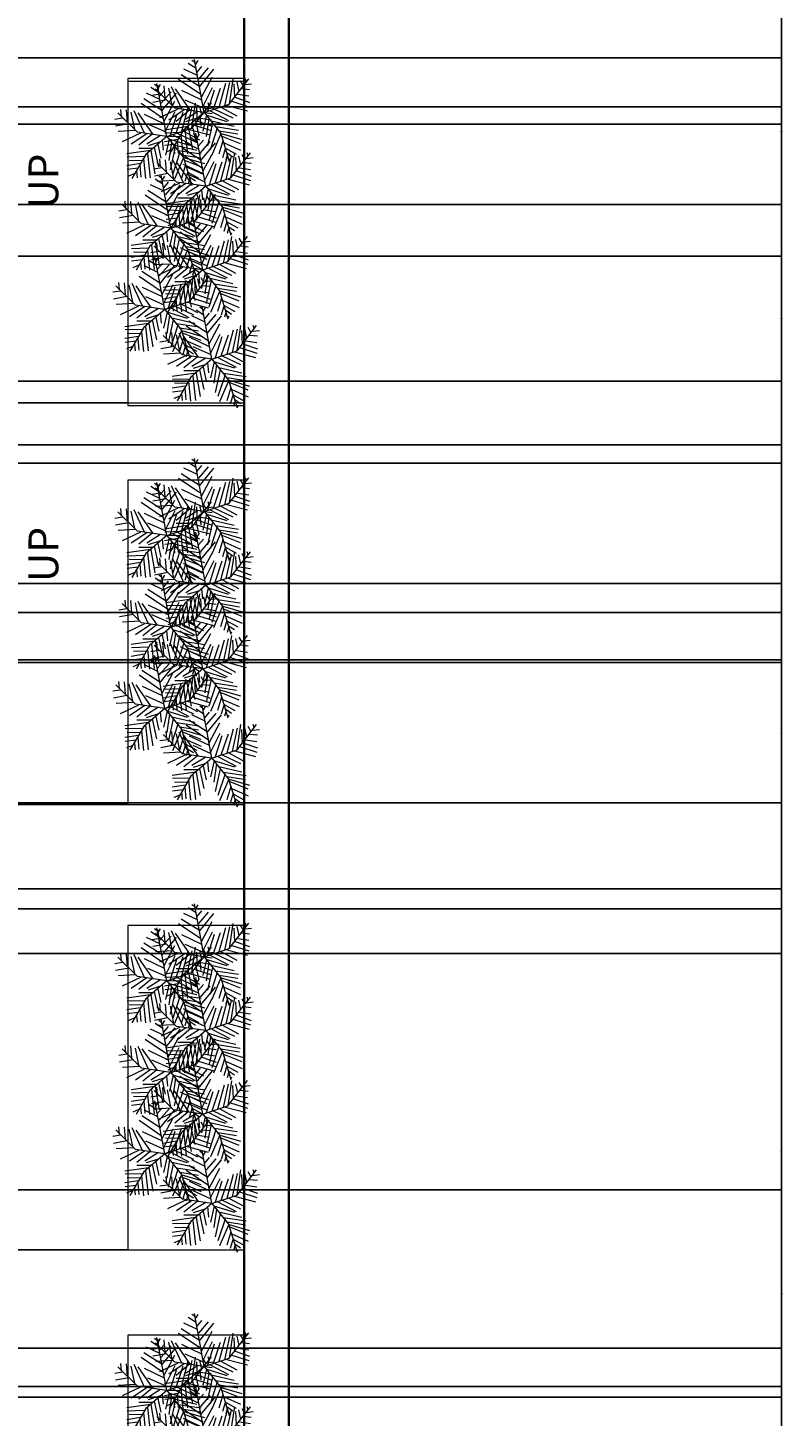
# Model space of a CAD drawing. Units: inches. Extents: x 818 to 1898, y 976 to 2364.
# Tile 56 of 96: x 1746 to 1898, y 1594 to 1873. Entities that reach past the tile are written whole.
import ezdxf

# ---------------------------------------------------------------- set-up
doc = ezdxf.new("R2010")
doc.units = ezdxf.units.IN
doc.header["$LTSCALE"] = 5
doc.header["$MEASUREMENT"] = 0
for name, color, linetype, lineweight in [('A-ANNO-DIMS', 2, 'Continuous', 18), ('A-ANNO-TEXT', 7, 'Continuous', 18), ('C-PROP', 7, 'Continuous', 35), ('L-PLNT-BEDS', 94, 'Continuous', 18)]:
    doc.layers.add(name, color=color, linetype=linetype, lineweight=lineweight)
doc.layers.add('L-PLNT', color=116, linetype='Continuous', lineweight=13, true_color=0x136734)
doc.styles.get("Standard").update_dxf_attribs({"font": 'arial.ttf'})
doc.dimstyles.get("Standard").update_dxf_attribs({"dimtxt": 0.18, "dimasz": 0.18, "dimexe": 0.18, "dimexo": 0.0625, "dimgap": 0.09, "dimtad": 0, "dimtih": 1, "dimtoh": 1, "dimdec": 4, "dimzin": 0, "dimdsep": 46, "dimtxsty": 'Standard', "dimcen": 0.09, "dimadec": 0, "dimazin": 0, "dimtfac": 1, "dimtdec": 4, "dimtofl": 0, "dimtmove": 0, "dimatfit": 3, "dimfxl": 1, "dimtolj": 1, "dimtzin": 0, "dimarcsym": 0})

# ---------------------------------------------------------------- blocks, each defined once
blk = doc.blocks.new('SHRUB-ACCENT')
for p, q in [((8.8, 18.63), (7.25, 19.67)), ((8.53, 19.84), (7.99, 20.28)), ((10.44, 9.82), (8.47, 20.47)), ((8.74, 19.5), (9.21, 20.28)), ((9.48, 15.07), (5.82, 17.41)), ((9.08, 17.24), (6.37, 18.54)), ((9.01, 17.93), (9.96, 19.06)), ((9.35, 16.54), (11.31, 18.8)), ((9.48, 14.98), (12.39, 18.54)), ((9.89, 12.9), (12.06, 16.89)), ((4.55, 10.66), (0.62, 14.58)), ((1.35, 13.77), (1.22, 15.24)), ((2.3, 15.16), (2.51, 12.72)), ((3.25, 14.72), (3.93, 11.25)), ((3.79, 15.07), (5.89, 10.55)), ((7.72, 10.21), (4.67, 14.55)), ((9.75, 13.42), (5.28, 16.46)), ((5.89, 14.29), (9.89, 12.38)), ((10.23, 11.07), (12.12, 14.81)), ((11.17, 10.12), (12.53, 14.37)), ((12.33, 10.47), (13.75, 14.72)), ((13.48, 10.9), (14.76, 15.68)), ((14.56, 11.16), (15.58, 15.85)), ((15.49, 11.5), (19.41, 16.55)), ((15.51, 11.51), (16.25, 16.54)), ((16.39, 15.59), (16.53, 12.9)), ((17, 15.94), (17.41, 14.03)), ((17.68, 16.2), (18.29, 15.16)), ((18.02, 14.63), (19.57, 14.46)), ((18.62, 15.42), (19.98, 15.59)), ((18.69, 16.63), (18.9, 15.94)), ((1.56, 13.51), (0, 13.25)), ((2.84, 12.38), (0.14, 11.86)), ((6.57, 12.38), (10.23, 10.73)), ((10.44, 9.82), (15.49, 11.5)), ((14.97, 11.25), (19.17, 10.12)), ((15.98, 12.12), (19.44, 10.99)), ((16.66, 12.9), (19.57, 11.86)), ((17.2, 13.51), (19.44, 13.16)), ((4.2, 10.99), (0.68, 10.81)), ((5.15, 10.47), (1.49, 8.73)), ((6.43, 10.38), (3.32, 8.3)), ((10.44, 9.82), (4.55, 10.66)), ((7.45, 10.21), (4.81, 8.04)), ((10.44, 9.82), (6.23, 6.17)), ((9.21, 10.03), (6.43, 8.3)), ((9.21, 8.73), (6.7, 7.95)), ((9.55, 9.16), (9.75, 7.08)), ((10.9, 9.25), (10.16, 6.04)), ((10.44, 9.82), (13.8, 5.61)), ((10.77, 9.34), (14.97, 8.04)), ((11.38, 8.64), (10.84, 5)), ((11.65, 10.12), (15.31, 8.21)), ((12.53, 10.47), (16.19, 8.73)), ((13.82, 10.9), (17, 9.16)), ((7.18, 6.99), (2.44, 6.3)), ((5.89, 5.78), (2.51, 5.69)), ((6.23, 6.17), (3.43, 1.4)), ((7.59, 7.43), (4.81, 7.43)), ((6.57, 6.39), (7.11, 1.52)), ((7.25, 6.99), (8.06, 2.31)), ((7.92, 7.69), (8.8, 3.69)), ((8.67, 8.21), (9.28, 5.43)), ((12.12, 7.69), (11.11, 3.09)), ((13.07, 6.65), (11.65, 2.31)), ((11.85, 8.12), (16.46, 7.08)), ((13.82, 5.6), (11.99, 1.26)), ((12.73, 6.99), (17.34, 6.3)), ((13.48, 6.13), (17.2, 5.52)), ((13.8, 5.61), (15.49, 0)), ((13.88, 5.6), (18.02, 4.39)), ((5.15, 4.39), (2.44, 3.95)), ((4.67, 3.43), (2.51, 3.17)), ((5.42, 4.91), (2.91, 5)), ((4.33, 2.91), (4.47, 1.52)), ((5.01, 4.04), (5.21, 1.61)), ((5.76, 5.34), (6.16, 1.35)), ((14.22, 4.13), (13.41, 1.44)), ((14.02, 5.08), (17.68, 3.61)), ((14.43, 3.69), (17.74, 2.22)), ((4, 2.39), (2.78, 1.87)), ((14.7, 2.74), (14.09, 0.74)), ((14.7, 2.65), (16.86, 1.44)), ((15.04, 1.26), (14.76, 0.31)), ((15.04, 1.7), (16.19, 0.92)), ((15.44, 0.48), (15.71, 0.31))]:
    blk.add_line(p, q)
blk = doc.blocks.new('PLANTER-RECT')
at = {"ltscale": 5}
blk.add_lwpolyline([(23.37, 65.17), (0, 65.17), (0, 0), (23.37, 0)], close=True, dxfattribs=at)
blk = doc.blocks.new('*D71')
at = {"layer": 'A-ANNO-DIMS', "color": 0, "lineweight": -2, "ltscale": 5, "transparency": 16777216}
for p, q in [((1714.79, 2053.08), (1897.92, 2053.08)), ((1897.74, 2052.9), (1897.74, 1699.76)), ((1897.74, 1346.26), (1897.74, 1699.4)), ((1714.79, 1346.08), (1897.92, 1346.08))]:
    blk.add_line(p, q, dxfattribs=at)
at = {"layer": 'A-ANNO-DIMS', "color": 0, "ltscale": 5, "transparency": 16777216}
for points in [[(1897.71, 2052.9), (1897.77, 2052.9), (1897.74, 2053.08)], [(1897.71, 1346.26), (1897.77, 1346.26), (1897.74, 1346.08)]]:
    blk.add_solid(points, dxfattribs=at)
at = {"layer": 'Defpoints', "color": 0, "ltscale": 5, "transparency": 16777216}
for p in [(1714.73, 2053.08), (1897.74, 2053.08), (1714.73, 1346.08)]:
    blk.add_point(p, dxfattribs=at)
at = {"layer": 'A-ANNO-DIMS', "color": 0, "ltscale": 5, "transparency": 16777216, "insert": (1897.74, 1699.58), "char_height": 0.18, "attachment_point": 5}
blk.add_mtext('\\A1;707', dxfattribs=at)
blk = doc.blocks.new('*D75')
at = {"layer": 'A-ANNO-DIMS', "color": 0, "lineweight": -2, "ltscale": 5, "transparency": 16777216}
for p, q in [((1705.79, 1785.61), (1897.92, 1785.61)), ((1897.74, 1785.43), (1897.74, 1770.79)), ((1897.74, 1755.79), (1897.74, 1770.43)), ((1705.79, 1755.61), (1897.92, 1755.61))]:
    blk.add_line(p, q, dxfattribs=at)
at = {"layer": 'A-ANNO-DIMS', "color": 0, "ltscale": 5, "transparency": 16777216}
for points in [[(1897.71, 1785.43), (1897.77, 1785.43), (1897.74, 1785.61)], [(1897.71, 1755.79), (1897.77, 1755.79), (1897.74, 1755.61)]]:
    blk.add_solid(points, dxfattribs=at)
at = {"layer": 'Defpoints', "color": 0, "ltscale": 5, "transparency": 16777216}
for p in [(1705.73, 1785.61), (1705.73, 1755.61), (1897.74, 1755.61)]:
    blk.add_point(p, dxfattribs=at)
at = {"layer": 'A-ANNO-DIMS', "color": 0, "ltscale": 5, "transparency": 16777216, "insert": (1897.74, 1770.61), "char_height": 0.18, "attachment_point": 5}
blk.add_mtext('\\A1;30', dxfattribs=at)
blk = doc.blocks.new('*D76')
at = {"layer": 'A-ANNO-DIMS', "color": 0, "lineweight": -2, "ltscale": 5, "transparency": 16777216}
for p, q in [((1705.79, 1857.21), (1897.92, 1857.21)), ((1897.74, 1857.03), (1897.74, 1842.39)), ((1897.74, 1827.39), (1897.74, 1842.03)), ((1705.79, 1827.21), (1897.92, 1827.21))]:
    blk.add_line(p, q, dxfattribs=at)
at = {"layer": 'A-ANNO-DIMS', "color": 0, "ltscale": 5, "transparency": 16777216}
for points in [[(1897.71, 1857.03), (1897.77, 1857.03), (1897.74, 1857.21)], [(1897.71, 1827.39), (1897.77, 1827.39), (1897.74, 1827.21)]]:
    blk.add_solid(points, dxfattribs=at)
at = {"layer": 'Defpoints', "color": 0, "ltscale": 5, "transparency": 16777216}
for p in [(1705.73, 1857.21), (1897.74, 1857.21), (1705.73, 1827.21)]:
    blk.add_point(p, dxfattribs=at)
at = {"layer": 'A-ANNO-DIMS', "color": 0, "ltscale": 5, "transparency": 16777216, "insert": (1897.74, 1842.21), "char_height": 0.18, "attachment_point": 5}
blk.add_mtext('\\A1;30', dxfattribs=at)
blk = doc.blocks.new('*D85')
at = {"layer": 'A-ANNO-DIMS', "color": 0, "lineweight": -2, "ltscale": 5, "transparency": 16777216}
for p, q in [((1258.79, 2053.08), (1897.92, 2053.08)), ((1897.74, 2052.9), (1897.74, 1876.76)), ((1897.74, 1700.26), (1897.74, 1876.4)), ((1258.79, 1700.08), (1897.92, 1700.08))]:
    blk.add_line(p, q, dxfattribs=at)
at = {"layer": 'A-ANNO-DIMS', "color": 0, "ltscale": 5, "transparency": 16777216}
for points in [[(1897.71, 2052.9), (1897.77, 2052.9), (1897.74, 2053.08)], [(1897.71, 1700.26), (1897.77, 1700.26), (1897.74, 1700.08)]]:
    blk.add_solid(points, dxfattribs=at)
at = {"layer": 'Defpoints', "color": 0, "ltscale": 5, "transparency": 16777216}
for p in [(1258.73, 2053.08), (1897.74, 2053.08), (1258.73, 1700.08)]:
    blk.add_point(p, dxfattribs=at)
at = {"layer": 'A-ANNO-DIMS', "color": 0, "ltscale": 5, "transparency": 16777216, "insert": (1897.74, 1876.58), "char_height": 0.18, "attachment_point": 5}
blk.add_mtext('\\A1;353', dxfattribs=at)
blk = doc.blocks.new('*D118')
at = {"layer": 'A-ANNO-DIMS', "color": 0, "lineweight": -2, "ltscale": 5, "transparency": 16777216}
for p, q in [((1766.29, 1627.51), (818.03, 1627.51)), ((818.21, 1627.33), (818.21, 1586.53)), ((818.21, 1545.36), (818.21, 1586.16)), ((1766.29, 1545.18), (818.03, 1545.18))]:
    blk.add_line(p, q, dxfattribs=at)
at = {"layer": 'A-ANNO-DIMS', "color": 0, "ltscale": 5, "transparency": 16777216}
for points in [[(818.18, 1627.33), (818.24, 1627.33), (818.21, 1627.51)], [(818.18, 1545.36), (818.24, 1545.36), (818.21, 1545.18)]]:
    blk.add_solid(points, dxfattribs=at)
at = {"layer": 'Defpoints', "color": 0, "ltscale": 5, "transparency": 16777216}
for p in [(818.21, 1627.51), (1766.35, 1627.51), (1766.35, 1545.18)]:
    blk.add_point(p, dxfattribs=at)
at = {"layer": 'A-ANNO-DIMS', "color": 0, "ltscale": 5, "transparency": 16777216, "insert": (818.21, 1586.34), "char_height": 0.18, "attachment_point": 5}
blk.add_mtext('\\A1;82.32', dxfattribs=at)
blk = doc.blocks.new('*D119')
at = {"layer": 'A-ANNO-DIMS', "color": 0, "lineweight": -2, "ltscale": 5, "transparency": 16777216}
for p, q in [((1766.29, 1716.99), (818.03, 1716.99)), ((818.21, 1716.81), (818.21, 1672.43)), ((818.21, 1627.69), (818.21, 1672.06)), ((1766.29, 1627.51), (818.03, 1627.51))]:
    blk.add_line(p, q, dxfattribs=at)
at = {"layer": 'A-ANNO-DIMS', "color": 0, "ltscale": 5, "transparency": 16777216}
for points in [[(818.18, 1716.81), (818.24, 1716.81), (818.21, 1716.99)], [(818.18, 1627.69), (818.24, 1627.69), (818.21, 1627.51)]]:
    blk.add_solid(points, dxfattribs=at)
at = {"layer": 'Defpoints', "color": 0, "ltscale": 5, "transparency": 16777216}
for p in [(818.21, 1716.99), (1766.35, 1716.99), (1766.35, 1627.51)]:
    blk.add_point(p, dxfattribs=at)
at = {"layer": 'A-ANNO-DIMS', "color": 0, "ltscale": 5, "transparency": 16777216, "insert": (818.21, 1672.25), "char_height": 0.18, "attachment_point": 5}
blk.add_mtext('\\A1;89.48', dxfattribs=at)
blk = doc.blocks.new('*D120')
at = {"layer": 'A-ANNO-DIMS', "color": 0, "lineweight": -2, "ltscale": 5, "transparency": 16777216}
for p, q in [((1766.29, 1797.72), (818.03, 1797.72)), ((818.21, 1797.54), (818.21, 1757.53)), ((818.21, 1717.17), (818.21, 1757.17)), ((1766.29, 1716.99), (818.03, 1716.99))]:
    blk.add_line(p, q, dxfattribs=at)
at = {"layer": 'A-ANNO-DIMS', "color": 0, "ltscale": 5, "transparency": 16777216}
for points in [[(818.18, 1797.54), (818.24, 1797.54), (818.21, 1797.72)], [(818.18, 1717.17), (818.24, 1717.17), (818.21, 1716.99)]]:
    blk.add_solid(points, dxfattribs=at)
at = {"layer": 'Defpoints', "color": 0, "ltscale": 5, "transparency": 16777216}
for p in [(818.21, 1797.72), (1766.35, 1797.72), (1766.35, 1716.99)]:
    blk.add_point(p, dxfattribs=at)
at = {"layer": 'A-ANNO-DIMS', "color": 0, "ltscale": 5, "transparency": 16777216, "insert": (818.21, 1757.35), "char_height": 0.18, "attachment_point": 5}
blk.add_mtext('\\A1;80.73', dxfattribs=at)
blk = doc.blocks.new('*D121')
at = {"layer": 'A-ANNO-DIMS', "color": 0, "lineweight": -2, "ltscale": 5, "transparency": 16777216}
for p, q in [((1766.29, 1884.2), (818.03, 1884.2)), ((818.21, 1884.02), (818.21, 1841.14)), ((818.21, 1797.9), (818.21, 1840.78)), ((1766.29, 1797.72), (818.03, 1797.72))]:
    blk.add_line(p, q, dxfattribs=at)
at = {"layer": 'A-ANNO-DIMS', "color": 0, "ltscale": 5, "transparency": 16777216}
for points in [[(818.18, 1884.02), (818.24, 1884.02), (818.21, 1884.2)], [(818.18, 1797.9), (818.24, 1797.9), (818.21, 1797.72)]]:
    blk.add_solid(points, dxfattribs=at)
at = {"layer": 'Defpoints', "color": 0, "ltscale": 5, "transparency": 16777216}
for p in [(818.21, 1884.2), (1766.35, 1884.2), (1766.35, 1797.72)]:
    blk.add_point(p, dxfattribs=at)
at = {"layer": 'A-ANNO-DIMS', "color": 0, "ltscale": 5, "transparency": 16777216, "insert": (818.21, 1840.96), "char_height": 0.18, "attachment_point": 5}
blk.add_mtext('\\A1;86.49', dxfattribs=at)
blk = doc.blocks.new('*D170')
at = {"layer": 'A-ANNO-DIMS', "color": 0, "lineweight": -2, "ltscale": 5, "transparency": 16777216}
for p, q in [((1430.79, 1600.08), (1897.92, 1600.08)), ((1897.74, 1599.9), (1897.74, 1550.76)), ((1897.74, 1501.26), (1897.74, 1550.4)), ((1430.79, 1501.08), (1897.92, 1501.08))]:
    blk.add_line(p, q, dxfattribs=at)
at = {"layer": 'A-ANNO-DIMS', "color": 0, "ltscale": 5, "transparency": 16777216}
for points in [[(1897.71, 1599.9), (1897.77, 1599.9), (1897.74, 1600.08)], [(1897.71, 1501.26), (1897.77, 1501.26), (1897.74, 1501.08)]]:
    blk.add_solid(points, dxfattribs=at)
at = {"layer": 'Defpoints', "color": 0, "ltscale": 5, "transparency": 16777216}
for p in [(1430.73, 1600.08), (1897.74, 1600.08), (1430.73, 1501.08)]:
    blk.add_point(p, dxfattribs=at)
at = {"layer": 'A-ANNO-DIMS', "color": 0, "ltscale": 5, "transparency": 16777216, "insert": (1897.74, 1550.58), "char_height": 0.18, "attachment_point": 5}
blk.add_mtext('\\A1;99', dxfattribs=at)
blk = doc.blocks.new('*D179')
at = {"layer": 'A-ANNO-DIMS', "color": 0, "lineweight": -2, "ltscale": 5, "transparency": 16777216}
for p, q in [((1669.79, 1687.08), (1897.92, 1687.08)), ((1897.74, 1686.9), (1897.74, 1643.76)), ((1897.74, 1600.26), (1897.74, 1643.4)), ((1669.79, 1600.08), (1897.92, 1600.08))]:
    blk.add_line(p, q, dxfattribs=at)
at = {"layer": 'A-ANNO-DIMS', "color": 0, "ltscale": 5, "transparency": 16777216}
for points in [[(1897.71, 1686.9), (1897.77, 1686.9), (1897.74, 1687.08)], [(1897.71, 1600.26), (1897.77, 1600.26), (1897.74, 1600.08)]]:
    blk.add_solid(points, dxfattribs=at)
at = {"layer": 'Defpoints', "color": 0, "ltscale": 5, "transparency": 16777216}
for p in [(1669.73, 1687.08), (1897.74, 1687.08), (1669.73, 1600.08)]:
    blk.add_point(p, dxfattribs=at)
at = {"layer": 'A-ANNO-DIMS', "color": 0, "ltscale": 5, "transparency": 16777216, "insert": (1897.74, 1643.58), "char_height": 0.18, "attachment_point": 5}
blk.add_mtext('\\A1;87', dxfattribs=at)
blk = doc.blocks.new('*D185')
at = {"layer": 'A-ANNO-DIMS', "color": 0, "lineweight": -2, "ltscale": 5, "transparency": 16777216}
for p, q in [((1737.9, 1639.58), (1897.92, 1639.58)), ((1897.74, 1639.4), (1897.74, 1618.93)), ((1897.74, 1598.1), (1897.74, 1618.57)), ((1737.9, 1597.92), (1897.92, 1597.92))]:
    blk.add_line(p, q, dxfattribs=at)
at = {"layer": 'A-ANNO-DIMS', "color": 0, "ltscale": 5, "transparency": 16777216}
for points in [[(1897.71, 1639.4), (1897.77, 1639.4), (1897.74, 1639.58)], [(1897.71, 1598.1), (1897.77, 1598.1), (1897.74, 1597.92)]]:
    blk.add_solid(points, dxfattribs=at)
at = {"layer": 'Defpoints', "color": 0, "ltscale": 5, "transparency": 16777216}
for p in [(1737.84, 1639.58), (1897.74, 1639.58), (1737.84, 1597.92)]:
    blk.add_point(p, dxfattribs=at)
at = {"layer": 'A-ANNO-DIMS', "color": 0, "ltscale": 5, "transparency": 16777216, "insert": (1897.74, 1618.75), "char_height": 0.18, "attachment_point": 5}
blk.add_mtext('\\A1;41.66', dxfattribs=at)
blk = doc.blocks.new('*D199')
at = {"layer": 'A-ANNO-DIMS', "color": 0, "lineweight": -2, "ltscale": 5, "transparency": 16777216}
for p, q in [((1559.79, 1687.08), (1897.92, 1687.08)), ((1897.74, 1686.9), (1897.74, 1513.15)), ((1897.74, 1339.05), (1897.74, 1512.79)), ((1660.38, 1338.87), (1897.92, 1338.87))]:
    blk.add_line(p, q, dxfattribs=at)
at = {"layer": 'A-ANNO-DIMS', "color": 0, "ltscale": 5, "transparency": 16777216}
for points in [[(1897.71, 1686.9), (1897.77, 1686.9), (1897.74, 1687.08)], [(1897.71, 1339.05), (1897.77, 1339.05), (1897.74, 1338.87)]]:
    blk.add_solid(points, dxfattribs=at)
at = {"layer": 'Defpoints', "color": 0, "ltscale": 5, "transparency": 16777216}
for p in [(1559.73, 1687.08), (1897.74, 1687.08), (1660.31, 1338.87)]:
    blk.add_point(p, dxfattribs=at)
at = {"layer": 'A-ANNO-DIMS', "color": 0, "ltscale": 5, "transparency": 16777216, "insert": (1897.74, 1512.97), "char_height": 0.18, "attachment_point": 5}
blk.add_mtext('\\A1;348.2', dxfattribs=at)
blk = doc.blocks.new('*D204')
at = {"layer": 'A-ANNO-DIMS', "color": 0, "lineweight": -2, "ltscale": 5, "transparency": 16777216}
for p, q in [((1714.79, 2053.08), (1897.92, 2053.08)), ((1897.74, 2052.9), (1897.74, 1960.26)), ((1897.74, 1867.26), (1897.74, 1959.9)), ((1705.79, 1867.08), (1897.92, 1867.08))]:
    blk.add_line(p, q, dxfattribs=at)
at = {"layer": 'A-ANNO-DIMS', "color": 0, "ltscale": 5, "transparency": 16777216}
for points in [[(1897.71, 2052.9), (1897.77, 2052.9), (1897.74, 2053.08)], [(1897.71, 1867.26), (1897.77, 1867.26), (1897.74, 1867.08)]]:
    blk.add_solid(points, dxfattribs=at)
at = {"layer": 'Defpoints', "color": 0, "ltscale": 5, "transparency": 16777216}
for p in [(1714.73, 2053.08), (1897.74, 2053.08), (1705.73, 1867.08)]:
    blk.add_point(p, dxfattribs=at)
at = {"layer": 'A-ANNO-DIMS', "color": 0, "ltscale": 5, "transparency": 16777216, "insert": (1897.74, 1960.08), "char_height": 0.18, "attachment_point": 5}
blk.add_mtext('\\A1;186', dxfattribs=at)
blk = doc.blocks.new('*D216')
at = {"layer": 'A-ANNO-DIMS', "color": 0, "lineweight": -2, "ltscale": 5, "transparency": 16777216}
for p, q in [((1705.79, 1717.32), (1897.92, 1717.32)), ((1897.74, 1717.14), (1897.74, 1706.88)), ((1897.74, 1696.26), (1897.74, 1706.52)), ((1705.79, 1696.08), (1897.92, 1696.08))]:
    blk.add_line(p, q, dxfattribs=at)
at = {"layer": 'A-ANNO-DIMS', "color": 0, "ltscale": 5, "transparency": 16777216}
for points in [[(1897.71, 1717.14), (1897.77, 1717.14), (1897.74, 1717.32)], [(1897.71, 1696.26), (1897.77, 1696.26), (1897.74, 1696.08)]]:
    blk.add_solid(points, dxfattribs=at)
at = {"layer": 'Defpoints', "color": 0, "ltscale": 5, "transparency": 16777216}
for p in [(1705.73, 1717.32), (1897.74, 1717.32), (1705.73, 1696.08)]:
    blk.add_point(p, dxfattribs=at)
at = {"layer": 'A-ANNO-DIMS', "color": 0, "ltscale": 5, "transparency": 16777216, "insert": (1897.74, 1706.7), "char_height": 0.18, "attachment_point": 5}
blk.add_mtext('\\A1;21.24', dxfattribs=at)
blk = doc.blocks.new('*D217')
at = {"layer": 'A-ANNO-DIMS', "color": 0, "lineweight": -2, "ltscale": 5, "transparency": 16777216}
for p, q in [((1705.79, 1745.56), (1897.92, 1745.56)), ((1897.74, 1745.38), (1897.74, 1731.62)), ((1897.74, 1717.5), (1897.74, 1731.26)), ((1705.79, 1717.32), (1897.92, 1717.32))]:
    blk.add_line(p, q, dxfattribs=at)
at = {"layer": 'A-ANNO-DIMS', "color": 0, "ltscale": 5, "transparency": 16777216}
for points in [[(1897.71, 1745.38), (1897.77, 1745.38), (1897.74, 1745.56)], [(1897.71, 1717.5), (1897.77, 1717.5), (1897.74, 1717.32)]]:
    blk.add_solid(points, dxfattribs=at)
at = {"layer": 'Defpoints', "color": 0, "ltscale": 5, "transparency": 16777216}
for p in [(1705.73, 1745.56), (1897.74, 1745.56), (1705.73, 1717.32)]:
    blk.add_point(p, dxfattribs=at)
at = {"layer": 'A-ANNO-DIMS', "color": 0, "ltscale": 5, "transparency": 16777216, "insert": (1897.74, 1731.44), "char_height": 0.18, "attachment_point": 5}
blk.add_mtext('\\A1;28.24', dxfattribs=at)
blk = doc.blocks.new('*D218')
at = {"layer": 'A-ANNO-DIMS', "color": 0, "lineweight": -2, "ltscale": 5, "transparency": 16777216}
for p, q in [((1705.79, 1827.21), (1897.92, 1827.21)), ((1897.74, 1827.03), (1897.74, 1814.83)), ((1897.74, 1802.26), (1897.74, 1814.46)), ((1705.79, 1802.08), (1897.92, 1802.08))]:
    blk.add_line(p, q, dxfattribs=at)
at = {"layer": 'A-ANNO-DIMS', "color": 0, "ltscale": 5, "transparency": 16777216}
for points in [[(1897.71, 1827.03), (1897.77, 1827.03), (1897.74, 1827.21)], [(1897.71, 1802.26), (1897.77, 1802.26), (1897.74, 1802.08)]]:
    blk.add_solid(points, dxfattribs=at)
at = {"layer": 'Defpoints', "color": 0, "ltscale": 5, "transparency": 16777216}
for p in [(1705.73, 1827.21), (1897.74, 1827.21), (1705.73, 1802.08)]:
    blk.add_point(p, dxfattribs=at)
at = {"layer": 'A-ANNO-DIMS', "color": 0, "ltscale": 5, "transparency": 16777216, "insert": (1897.74, 1814.65), "char_height": 0.18, "attachment_point": 5}
blk.add_mtext('\\A1;25.134', dxfattribs=at)
blk = doc.blocks.new('*D225')
at = {"layer": 'A-ANNO-DIMS', "color": 0, "lineweight": -2, "ltscale": 5, "transparency": 16777216}
for p, q in [((1532.66, 1867.08), (1897.92, 1867.08)), ((1897.74, 1866.9), (1897.74, 1852.51)), ((1897.74, 1837.76), (1897.74, 1852.15)), ((1532.66, 1837.58), (1897.92, 1837.58))]:
    blk.add_line(p, q, dxfattribs=at)
at = {"layer": 'A-ANNO-DIMS', "color": 0, "ltscale": 5, "transparency": 16777216}
for points in [[(1897.71, 1866.9), (1897.77, 1866.9), (1897.74, 1867.08)], [(1897.71, 1837.76), (1897.77, 1837.76), (1897.74, 1837.58)]]:
    blk.add_solid(points, dxfattribs=at)
at = {"layer": 'Defpoints', "color": 0, "ltscale": 5, "transparency": 16777216}
for p in [(1532.59, 1867.08), (1897.74, 1867.08), (1532.59, 1837.58)]:
    blk.add_point(p, dxfattribs=at)
at = {"layer": 'A-ANNO-DIMS', "color": 0, "ltscale": 5, "transparency": 16777216, "insert": (1897.74, 1852.33), "char_height": 0.18, "attachment_point": 5}
blk.add_mtext('\\A1;29.496', dxfattribs=at)
blk = doc.blocks.new('*D268')
at = {"layer": 'A-ANNO-DIMS', "color": 0, "lineweight": -2, "ltscale": 5, "transparency": 16777216}
for p, q in [((1741.9, 1890.29), (1897.92, 1890.29)), ((1897.74, 1890.11), (1897.74, 1788.87)), ((1897.74, 1687.26), (1897.74, 1788.5)), ((1741.9, 1687.08), (1897.92, 1687.08))]:
    blk.add_line(p, q, dxfattribs=at)
at = {"layer": 'A-ANNO-DIMS', "color": 0, "ltscale": 5, "transparency": 16777216}
for points in [[(1897.71, 1890.11), (1897.77, 1890.11), (1897.74, 1890.29)], [(1897.71, 1687.26), (1897.77, 1687.26), (1897.74, 1687.08)]]:
    blk.add_solid(points, dxfattribs=at)
at = {"layer": 'Defpoints', "color": 0, "ltscale": 5, "transparency": 16777216}
for p in [(1741.84, 1890.29), (1897.74, 1890.29), (1741.84, 1687.08)]:
    blk.add_point(p, dxfattribs=at)
at = {"layer": 'A-ANNO-DIMS', "color": 0, "ltscale": 5, "transparency": 16777216, "insert": (1897.74, 1788.68), "char_height": 0.18, "attachment_point": 5}
blk.add_mtext('\\A1;203.2', dxfattribs=at)
blk = doc.blocks.new('*D275')
at = {"layer": 'A-ANNO-DIMS', "color": 0, "lineweight": -2, "ltscale": 5, "transparency": 16777216}
for p, q in [((1377.84, 1897.87), (1897.92, 1897.87)), ((1897.74, 1897.69), (1897.74, 1875.99)), ((1897.74, 1853.93), (1897.74, 1875.63)), ((1377.84, 1853.75), (1897.92, 1853.75))]:
    blk.add_line(p, q, dxfattribs=at)
at = {"layer": 'A-ANNO-DIMS', "color": 0, "ltscale": 5, "transparency": 16777216}
for points in [[(1897.71, 1897.69), (1897.77, 1897.69), (1897.74, 1897.87)], [(1897.71, 1853.93), (1897.77, 1853.93), (1897.74, 1853.75)]]:
    blk.add_solid(points, dxfattribs=at)
at = {"layer": 'Defpoints', "color": 0, "ltscale": 5, "transparency": 16777216}
for p in [(1377.78, 1897.87), (1897.74, 1897.87), (1377.78, 1853.75)]:
    blk.add_point(p, dxfattribs=at)
at = {"layer": 'A-ANNO-DIMS', "color": 0, "ltscale": 5, "transparency": 16777216, "insert": (1897.74, 1875.81), "char_height": 0.18, "attachment_point": 5}
blk.add_mtext('\\A1;44.12', dxfattribs=at)
blk = doc.blocks.new('*D280')
at = {"layer": 'A-ANNO-DIMS', "color": 0, "lineweight": -2, "ltscale": 5, "transparency": 16777216}
for p, q in [((1398.73, 1789.31), (1897.92, 1789.31)), ((1897.74, 1789.13), (1897.74, 1767.89)), ((1897.74, 1746.29), (1897.74, 1767.53)), ((1397.41, 1746.11), (1897.92, 1746.11))]:
    blk.add_line(p, q, dxfattribs=at)
at = {"layer": 'A-ANNO-DIMS', "color": 0, "ltscale": 5, "transparency": 16777216}
for points in [[(1897.71, 1789.13), (1897.77, 1789.13), (1897.74, 1789.31)], [(1897.71, 1746.29), (1897.77, 1746.29), (1897.74, 1746.11)]]:
    blk.add_solid(points, dxfattribs=at)
at = {"layer": 'Defpoints', "color": 0, "ltscale": 5, "transparency": 16777216}
for p in [(1398.67, 1789.31), (1897.74, 1789.31), (1397.35, 1746.11)]:
    blk.add_point(p, dxfattribs=at)
at = {"layer": 'A-ANNO-DIMS', "color": 0, "ltscale": 5, "transparency": 16777216, "insert": (1897.74, 1767.71), "char_height": 0.18, "attachment_point": 5}
blk.add_mtext('\\A1;43.19', dxfattribs=at)
blk = doc.blocks.new('*D282')
at = {"layer": 'A-ANNO-DIMS', "color": 0, "lineweight": -2, "ltscale": 5, "transparency": 16777216}
for p, q in [((1422.08, 2081.19), (1897.92, 2081.19)), ((1897.74, 2081.01), (1897.74, 1884.32)), ((1897.74, 1687.26), (1897.74, 1883.95)), ((1463.79, 1687.08), (1897.92, 1687.08))]:
    blk.add_line(p, q, dxfattribs=at)
at = {"layer": 'A-ANNO-DIMS', "color": 0, "ltscale": 5, "transparency": 16777216}
for points in [[(1897.71, 2081.01), (1897.77, 2081.01), (1897.74, 2081.19)], [(1897.71, 1687.26), (1897.77, 1687.26), (1897.74, 1687.08)]]:
    blk.add_solid(points, dxfattribs=at)
at = {"layer": 'Defpoints', "color": 0, "ltscale": 5, "transparency": 16777216}
for p in [(1422.02, 2081.19), (1897.74, 2081.19), (1463.73, 1687.08)]:
    blk.add_point(p, dxfattribs=at)
at = {"layer": 'A-ANNO-DIMS', "color": 0, "ltscale": 5, "transparency": 16777216, "insert": (1897.74, 1884.13), "char_height": 0.18, "attachment_point": 5}
blk.add_mtext('\\A1;394.1', dxfattribs=at)
blk = doc.blocks.new('*D284')
at = {"layer": 'A-ANNO-DIMS', "color": 0, "lineweight": -2, "ltscale": 5, "transparency": 16777216}
for p, q in [((1351.66, 1761.45), (1897.92, 1761.45)), ((1897.74, 1761.27), (1897.74, 1728.95)), ((1897.74, 1696.26), (1897.74, 1728.58)), ((1267.79, 1696.08), (1897.92, 1696.08))]:
    blk.add_line(p, q, dxfattribs=at)
at = {"layer": 'A-ANNO-DIMS', "color": 0, "ltscale": 5, "transparency": 16777216}
for points in [[(1897.71, 1761.27), (1897.77, 1761.27), (1897.74, 1761.45)], [(1897.71, 1696.26), (1897.77, 1696.26), (1897.74, 1696.08)]]:
    blk.add_solid(points, dxfattribs=at)
at = {"layer": 'Defpoints', "color": 0, "ltscale": 5, "transparency": 16777216}
for p in [(1351.6, 1761.45), (1267.73, 1696.08), (1897.74, 1696.08)]:
    blk.add_point(p, dxfattribs=at)
at = {"layer": 'A-ANNO-DIMS', "color": 0, "ltscale": 5, "transparency": 16777216, "insert": (1897.74, 1728.76), "char_height": 0.18, "attachment_point": 5}
blk.add_mtext('\\A1;65.37', dxfattribs=at)
blk = doc.blocks.new('*D291')
at = {"layer": 'A-ANNO-DIMS', "color": 0, "lineweight": -2, "ltscale": 5, "transparency": 16777216}
for p, q in [((1206.79, 1687.08), (1897.92, 1687.08)), ((1897.74, 1686.9), (1897.74, 1647.61)), ((1897.74, 1607.95), (1897.74, 1647.24)), ((1318.96, 1607.77), (1897.92, 1607.77))]:
    blk.add_line(p, q, dxfattribs=at)
at = {"layer": 'A-ANNO-DIMS', "color": 0, "ltscale": 5, "transparency": 16777216}
for points in [[(1897.71, 1686.9), (1897.77, 1686.9), (1897.74, 1687.08)], [(1897.71, 1607.95), (1897.77, 1607.95), (1897.74, 1607.77)]]:
    blk.add_solid(points, dxfattribs=at)
at = {"layer": 'Defpoints', "color": 0, "ltscale": 5, "transparency": 16777216}
for p in [(1206.73, 1687.08), (1897.74, 1687.08), (1318.89, 1607.77)]:
    blk.add_point(p, dxfattribs=at)
at = {"layer": 'A-ANNO-DIMS', "color": 0, "ltscale": 5, "transparency": 16777216, "insert": (1897.74, 1647.42), "char_height": 0.18, "attachment_point": 5}
blk.add_mtext('\\A1;79.3', dxfattribs=at)

msp = doc.modelspace()

# ---------------------------------------------------------------- linework, layer by layer
at = {"layer": 'C-PROP', "ltscale": 5}
for p, q in [((1798.7173, 1202.9642), (1798.7173, 2294.2171)), ((1789.7173, 1211.9642), (1789.7173, 2285.2171))]:
    msp.add_line(p, q, dxfattribs=at)

# ---------------------------------------------------------------- block references
at = {"layer": 'L-PLNT'}
for p in [(1771.257, 1846.2506), (1763.7314, 1841.4317), (1771.5761, 1831.4236), (1764.5652, 1823.0105), (1770.9913, 1814.6319), (1763.3302, 1806.6873), (1772.8128, 1796.7014), (1771.257, 1766.0765), (1763.7314, 1761.2577), (1771.5761, 1751.2496), (1764.5652, 1742.8365), (1770.9913, 1734.4578), (1763.3302, 1726.5132), (1772.8128, 1716.5273), (1771.257, 1676.5951), (1763.7314, 1671.7763), (1771.5761, 1661.7682), (1764.5652, 1653.3551), (1770.9913, 1644.9764), (1763.3302, 1637.0318), (1772.8128, 1627.0459), (1771.257, 1594.2726), (1763.7314, 1589.4538), (1771.5761, 1579.4457)]:
    msp.add_blockref('SHRUB-ACCENT', p, dxfattribs=at)
at = {"layer": 'L-PLNT-BEDS'}
for p in [(1766.352, 1797.7165), (1766.352, 1797.1606), (1766.352, 1716.9865), (1766.352, 1716.9865), (1766.352, 1627.5051), (1766.352, 1627.5051), (1766.352, 1545.1826), (1766.352, 1545.1826)]:
    msp.add_blockref('PLANTER-RECT', p, dxfattribs=at)

# ---------------------------------------------------------------- texts
at = {"layer": 'A-ANNO-TEXT', "ltscale": 5, "char_height": 6, "attachment_point": 1, "rotation": 90}
for insert in [(1746.3735, 1836.7106), (1746.3735, 1761.705)]:
    msp.add_mtext_dynamic_manual_height_columns('UP', width=118.992422, gutter_width=1, heights=[0], dxfattribs=dict(at, insert=insert))

# ---------------------------------------------------------------- dimensions: what is measured, and where the dimension line sits
at = {"layer": 'A-ANNO-DIMS', "ltscale": 5}
for base, p1, p2, override, picture, middle in [((1897.736, 2081.1881), (1463.7251, 1687.0782), (1422.02, 2081.1881), {"dimdec": 1, "dimlfac": 1, "dimrnd": 0, "dimzin": 0, "dimdsep": 46, "dimlunit": 2}, '*D282', (1897.736, 1884.1332)), ((1897.736, 2053.0782), (1258.7251, 1700.0782), (1258.7251, 2053.0782), {"dimdec": 0, "dimlfac": 1, "dimrnd": 0, "dimzin": 0, "dimdsep": 46, "dimlunit": 2}, '*D85', (1897.736, 1876.5782)), ((1897.736, 2053.0782), (1705.7251, 1867.0782), (1714.7251, 2053.0782), {"dimdec": 0, "dimlfac": 1, "dimrnd": 0, "dimzin": 0, "dimdsep": 46, "dimlunit": 2}, '*D204', (1897.736, 1960.0782)), ((1897.736, 2053.0782), (1714.7251, 1346.0782), (1714.7251, 2053.0782), {"dimdec": 0, "dimlfac": 1, "dimrnd": 0, "dimzin": 0, "dimdsep": 46, "dimlunit": 2}, '*D71', (1897.736, 1699.5782)), ((1897.736, 1897.8663), (1377.7791, 1853.7496), (1377.7791, 1897.8663), {"dimdec": 2, "dimlfac": 1, "dimrnd": 0, "dimzin": 0, "dimdsep": 46, "dimlunit": 2}, '*D275', (1897.736, 1875.808)), ((1897.736, 1890.2903), (1741.8409, 1687.0782), (1741.8409, 1890.2903), {"dimdec": 1, "dimlfac": 1, "dimrnd": 0, "dimzin": 0, "dimdsep": 46, "dimlunit": 2}, '*D268', (1897.736, 1788.6843)), ((818.2059, 1884.2031), (1766.3524, 1797.7165), (1766.3524, 1884.2031), {"dimdec": 2, "dimlfac": 1, "dimrnd": 0, "dimzin": 0, "dimdsep": 46, "dimlunit": 2}, '*D121', (818.2059, 1840.9598)), ((1897.736, 1867.0782), (1532.593, 1837.5823), (1532.593, 1867.0782), {"dimdec": 3, "dimlfac": 1, "dimrnd": 0, "dimzin": 0, "dimdsep": 46, "dimlunit": 2}, '*D225', (1897.736, 1852.3303)), ((1897.736, 1857.2125), (1705.7251, 1827.2125), (1705.7251, 1857.2125), {"dimdec": 0, "dimlfac": 1, "dimrnd": 0, "dimzin": 0, "dimdsep": 46, "dimlunit": 2}, '*D76', (1897.736, 1842.2125)), ((1897.736, 1827.2125), (1705.7251, 1802.0782), (1705.7251, 1827.2125), {"dimdec": 3, "dimlfac": 1, "dimrnd": 0, "dimzin": 0, "dimdsep": 46, "dimlunit": 2}, '*D218', (1897.736, 1814.6454)), ((818.2059, 1797.7165), (1766.3524, 1716.9866), (1766.3524, 1797.7165), {"dimdec": 2, "dimlfac": 1, "dimrnd": 0, "dimzin": 0, "dimdsep": 46, "dimlunit": 2}, '*D120', (818.2059, 1757.3516)), ((1897.736, 1789.3057), (1397.3459, 1746.1142), (1398.6717, 1789.3057), {"dimdec": 2, "dimlfac": 1, "dimrnd": 0, "dimzin": 0, "dimdsep": 46, "dimlunit": 2}, '*D280', (1897.736, 1767.71)), ((1897.736, 1755.6125), (1705.7251, 1785.6125), (1705.7251, 1755.6125), {"dimdec": 0, "dimlfac": 1, "dimrnd": 0, "dimzin": 0, "dimdsep": 46, "dimlunit": 2}, '*D75', (1897.736, 1770.6125)), ((1897.736, 1696.0782), (1351.5985, 1761.449), (1267.7251, 1696.0782), {"dimdec": 2, "dimlfac": 1, "dimrnd": 0, "dimzin": 0, "dimdsep": 46, "dimlunit": 2}, '*D284', (1897.736, 1728.7636)), ((1897.736, 1745.5584), (1705.7251, 1717.3178), (1705.7251, 1745.5584), {"dimdec": 2, "dimlfac": 1, "dimrnd": 0, "dimzin": 0, "dimdsep": 46, "dimlunit": 2}, '*D217', (1897.736, 1731.4381)), ((818.2059, 1716.9866), (1766.3524, 1627.5052), (1766.3524, 1716.9866), {"dimdec": 2, "dimlfac": 1, "dimrnd": 0, "dimzin": 0, "dimdsep": 46, "dimlunit": 2}, '*D119', (818.2059, 1672.2459)), ((1897.736, 1717.3178), (1705.7251, 1696.0782), (1705.7251, 1717.3178), {"dimdec": 2, "dimlfac": 1, "dimrnd": 0, "dimzin": 0, "dimdsep": 46, "dimlunit": 2}, '*D216', (1897.736, 1706.698)), ((1897.736, 1687.0782), (1318.8931, 1607.7707), (1206.7251, 1687.0782), {"dimdec": 1, "dimlfac": 1, "dimrnd": 0, "dimzin": 0, "dimdsep": 46, "dimlunit": 2}, '*D291', (1897.736, 1647.4245)), ((1897.736, 1687.0782), (1660.3141, 1338.8654), (1559.7251, 1687.0782), {"dimdec": 1, "dimlfac": 1, "dimrnd": 0, "dimzin": 0, "dimdsep": 46, "dimlunit": 2}, '*D199', (1897.736, 1512.9718)), ((1897.736, 1687.0782), (1669.7251, 1600.0782), (1669.7251, 1687.0782), {"dimdec": 0, "dimlfac": 1, "dimrnd": 0, "dimzin": 0, "dimdsep": 46, "dimlunit": 2}, '*D179', (1897.736, 1643.5782)), ((1897.736, 1639.5782), (1737.8409, 1597.9175), (1737.8409, 1639.5782), {"dimdec": 2, "dimlfac": 1, "dimrnd": 0, "dimzin": 0, "dimdsep": 46, "dimlunit": 2}, '*D185', (1897.736, 1618.7479)), ((818.2059, 1627.5052), (1766.3524, 1545.1827), (1766.3524, 1627.5052), {"dimdec": 2, "dimlfac": 1, "dimrnd": 0, "dimzin": 0, "dimdsep": 46, "dimlunit": 2}, '*D118', (818.2059, 1586.3439)), ((1897.736, 1600.0782), (1430.7251, 1501.0782), (1430.7251, 1600.0782), {"dimdec": 0, "dimlfac": 1, "dimrnd": 0, "dimzin": 0, "dimdsep": 46, "dimlunit": 2}, '*D170', (1897.736, 1550.5782))]:
    dim = msp.add_linear_dim(base=base, p1=p1, p2=p2, angle=90, dimstyle='Standard', override=override, dxfattribs=at)
    dim.commit()
    dim.dimension.update_dxf_attribs({"geometry": picture, "text_midpoint": middle})

doc.saveas('drawing.dxf')
